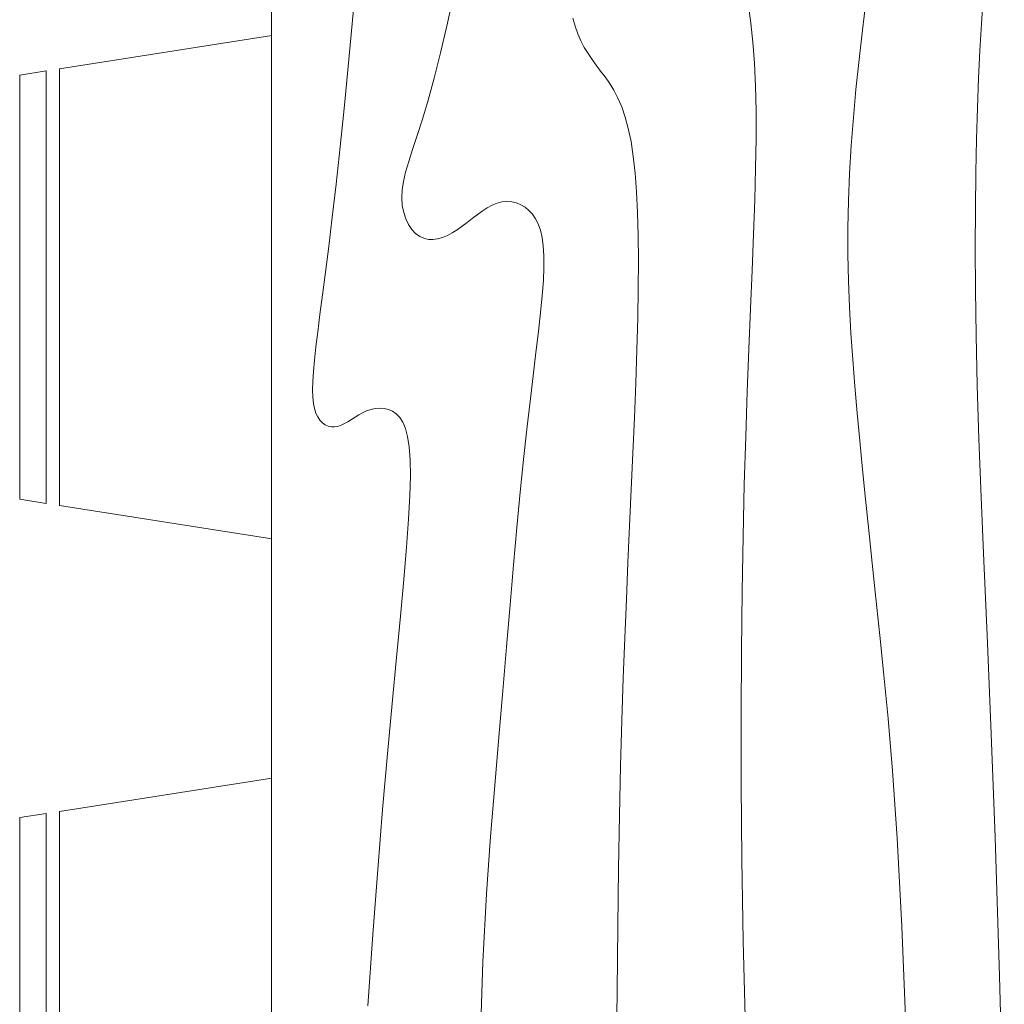
# Model space of a CAD drawing. Units: inches. Extents: x -301 to 715, y -607 to 364.
# Tile 110 of 141: x -41 to -13, y 147 to 175. Entities that reach past the tile are written whole.
import ezdxf

# ---------------------------------------------------------------- set-up
doc = ezdxf.new("R2010")
doc.units = ezdxf.units.IN
doc.header["$MEASUREMENT"] = 0
doc.layers.add('A-FURN', color=8, linetype='Continuous', lineweight=18)

# ---------------------------------------------------------------- blocks, each defined once
blk = doc.blocks.new('Dining Set - 36 x 72 in.')
for p, q in [((-22, 27.5), (-6, 27.5)), ((-5.8437, 26.49966), (-6, 27.5)), ((6, 27.5), (5.8438, 26.50042)), ((6, 27.5), (22, 27.5)), ((22.1563, 26.49966), (22, 27.5)), ((-5.8416, 26.5), (-22.1534, 26.5)), ((22.1584, 26.5), (5.8466, 26.5)), ((-22.2304, 26), (-5.7608, 26)), ((-4.5152, 17.99762), (-5.7655, 25.99926)), ((5.7657, 26.00059), (4.5153, 17.99762)), ((5.7696, 26), (22.2392, 26)), ((23.4848, 17.99762), (22.2345, 25.99926)), ((36, 18), (-36, 18))]:
    blk.add_line(p, q)
for points in [[(-13.0957, 14.36718), (-10.4159, 14.18652), (-7.9583, 14), (-5.6904, 13.81315), (-3.6035, 13.63021), (-1.6954, 13.45508), (0.0365, 13.29166), (1.5945, 13.14388), (2.9811, 13.01562), (4.1988, 12.9108), (5.25, 12.83333), (6.1393, 12.78613), (6.8802, 12.76823), (7.4883, 12.77767), (7.9792, 12.8125), (8.3685, 12.87077), (8.6719, 12.95052), (8.9049, 13.0498), (9.0833, 13.16666), (9.2205, 13.29899), (9.3216, 13.44401), (9.3895, 13.59879), (9.4271, 13.76041), (9.4373, 13.92594), (9.4232, 14.09245), (9.3875, 14.257), (9.3333, 14.41666), (9.2638, 14.56917), (9.1836, 14.71484), (9.0975, 14.85465), (9.0104, 14.98958), (8.9272, 15.1206), (8.8529, 15.2487), (8.7922, 15.37483), (8.75, 15.5), (8.7305, 15.62467), (8.7344, 15.74739), (8.7617, 15.86621), (8.8125, 15.97916), (8.8867, 16.08431), (8.9844, 16.17968), (9.1055, 16.26334), (9.25, 16.33333), (9.4189, 16.38802), (9.6172, 16.42708), (9.8506, 16.45052), (10.125, 16.45833), (10.4463, 16.45052), (10.8203, 16.42708), (11.2529, 16.38802), (11.75, 16.33333), (12.3184, 16.26318), (12.9694, 16.17838), (13.7151, 16.07991), (14.5677, 15.96875), (15.5395, 15.84586), (16.6426, 15.71224), (17.8893, 15.56884), (19.2917, 15.41666), (20.859, 15.25667), (22.5879, 15.08984), (24.4721, 14.91715)], [(-14.5677, 10.13541), (-11.4399, 10.03011), (-8.877, 9.89453), (-6.7154, 9.74137), (-4.7917, 9.58333), (-2.9698, 9.43082), (-1.2246, 9.28515), (0.4415, 9.14534), (2.026, 9.01041), (3.5266, 8.87939), (4.9408, 8.7513), (6.266, 8.62516), (7.5, 8.5), (8.6411, 8.37549), (9.6914, 8.2539), (10.6538, 8.13818), (11.5312, 8.03125), (12.3267, 7.93603), (13.043, 7.85547), (13.6831, 7.79248), (14.25, 7.75), (14.7471, 7.7303), (15.1797, 7.73307), (15.5537, 7.75732), (15.875, 7.80208), (16.1494, 7.86637), (16.3828, 7.94922), (16.5811, 8.04964), (16.75, 8.16666), (16.8944, 8.29915), (17.0143, 8.44531), (17.1089, 8.60319), (17.1771, 8.77083), (17.218, 8.94629), (17.2305, 9.1276), (17.2137, 9.31282), (17.1667, 9.5), (17.0895, 9.6875), (16.987, 9.875), (16.8649, 10.0625), (16.7292, 10.25), (16.5856, 10.4375), (16.4401, 10.625), (16.2985, 10.8125), (16.1667, 11), (16.05, 11.18733), (15.9518, 11.3737), (15.8752, 11.5581), (15.8229, 11.73958), (15.798, 11.91715), (15.8034, 12.08984), (15.842, 12.25667), (15.9167, 12.41666), (16.0295, 12.56836), (16.1784, 12.70833), (16.3605, 12.83268), (16.5729, 12.9375), (16.8127, 13.01888), (17.0768, 13.07291), (17.3625, 13.0957), (17.6667, 13.08333), (17.9894, 13.03312), (18.3418, 12.94726), (18.7382, 12.82918), (19.1927, 12.68229), (19.7195, 12.51001), (20.3327, 12.31575), (21.0465, 12.10294), (21.875, 11.875), (22.8357, 11.63354), (23.959, 11.37304), (25.2786, 11.08618)], [(-15.3009, 5.00602), (-12.5508, 4.97265), (-10.1112, 4.94515), (-7.9167, 4.91666), (-5.909, 4.88167), (-4.0586, 4.83984), (-2.3429, 4.79215), (-0.7396, 4.73958), (0.7739, 4.6831), (2.22, 4.6237), (3.6213, 4.56233), (5, 4.5), (6.373, 4.43782), (7.7344, 4.3776), (9.0723, 4.32129), (10.375, 4.27083), (11.6309, 4.22819), (12.8281, 4.19531), (13.9551, 4.17415), (15, 4.16666), (15.954, 4.17448), (16.819, 4.19791), (17.6001, 4.23698), (18.3021, 4.29166), (18.9299, 4.36198), (19.4883, 4.44791), (19.9823, 4.54948), (20.4167, 4.66666), (20.7969, 4.79899), (21.1302, 4.94401), (21.4245, 5.09879), (21.6875, 5.26041), (21.9271, 5.42594), (22.1511, 5.59245), (22.3672, 5.757), (22.5834, 5.91666), (22.8065, 6.06868), (23.0404, 6.21093), (23.2879, 6.34147), (23.5521, 6.45833), (23.8358, 6.55957), (24.142, 6.64323)], [(-14.0005, 0.12833), (-10.6523, 0.21289), (-7.5796, 0.26522), (-4.75, 0.29166), (-2.134, 0.29793), (0.2878, 0.28711), (2.5317, 0.26163), (4.6146, 0.22396), (6.5529, 0.17651), (8.3633, 0.12174), (10.0623, 0.06209), (11.6667, 0), (13.1899, -0.06201), (14.6341, -0.1211), (15.9982, -0.17432), (17.2813, -0.21875), (18.4823, -0.25147), (19.6003, -0.26953), (20.6343, -0.27002), (21.5834, -0.25), (22.4481, -0.20768), (23.2357, -0.14584), (23.9549, -0.06836), (24.6146, 0.02083)], [(-14.469, -5.9419), (-10.1094, -5.76042), (-6.7752, -5.58285), (-4.2363, -5.41016), (-2.2629, -5.24333), (-0.625, -5.08334), (0.8708, -4.93099), (2.2715, -4.78646), (3.5872, -4.64974), (4.8281, -4.52084), (6.0046, -4.39974), (7.127, -4.28646), (8.2053, -4.18099), (9.25, -4.08334), (10.2705, -3.99382), (11.2734, -3.91407), (12.2647, -3.84603), (13.25, -3.79167), (14.2354, -3.75293), (15.2266, -3.73177), (16.2295, -3.73015), (17.25, -3.75), (18.2912, -3.79248), (19.3451, -3.85547), (20.4009, -3.93604), (21.4479, -4.03125), (22.4754, -4.13819), (23.4727, -4.25391), (24.4289, -4.37549)], [(-18.4675, -9.62891), (-11.9839, -9.45069), (-6.7396, -9.28125), (-2.5226, -9.12354), (0.8789, -8.98047), (3.6769, -8.85498), (6.0833, -8.75), (8.2767, -8.66765), (10.3021, -8.60677), (12.1712, -8.56543), (13.8958, -8.54167), (15.4876, -8.53353), (16.9583, -8.53907), (18.3197, -8.55632), (19.5834, -8.58334), (20.7616, -8.61841), (21.8685, -8.66081), (22.9188, -8.71004), (23.9271, -8.76563), (24.9081, -8.82707)]]:
    blk.add_lwpolyline(points)

msp = doc.modelspace()

# ---------------------------------------------------------------- block references
at = {"layer": 'A-FURN', "xscale": 0.753207081168398, "yscale": 0.753207081168398, "zscale": 0.753207081168398, "rotation": 90}
msp.add_blockref('Dining Set - 36 x 72 in.', (-20.244, 157.036), dxfattribs=at)

doc.saveas('drawing.dxf')
